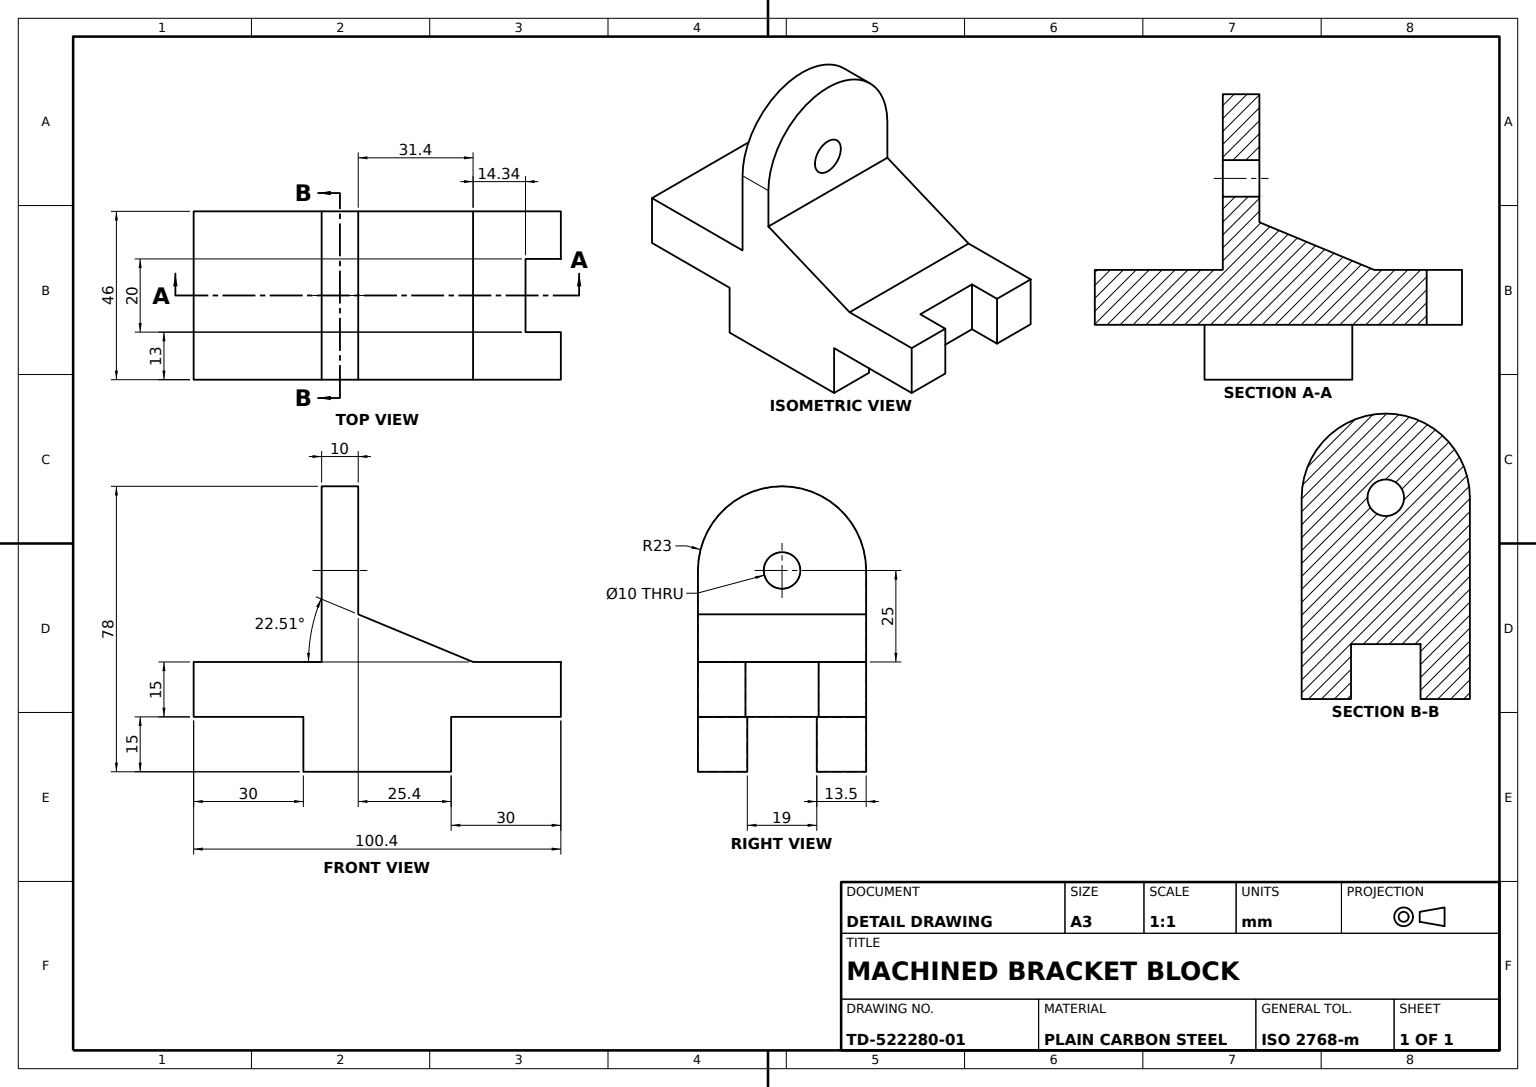
SolidWorks part; units mm, degrees
material "Plain Carbon Steel"
ref_plane "Front Plane" through (0, 0, 0) normal (0, 0, 1) x (1, 0, 0)
ref_plane "Top Plane" through (0, 0, 0) normal (0, 1, 0) x (1, 0, 0)
ref_plane "Right Plane" through (0, 0, 0) normal (1, 0, 0) x (0, 0, -1)
sketch "Base Profile Sketch" plane through (0, 0, 0) normal (1, 0, 0) x (0, 0, -1)
  line L0 (50.2023, 0) -> (-50.2023, 0)
  line L1 (-50.2023, 0) -> (-50.2023, -15)
  line L2 (-50.2023, -15) -> (-20.2023, -15)
  line L3 (-20.2023, -15) -> (-20.2023, -30)
  line L4 (50.2023, 0) -> (50.2023, -15)
  line L5 (50.2023, -15) -> (20.2023, -15)
  line L6 (20.2023, -15) -> (20.2023, -30)
  line L7 (20.2023, -30) -> (-20.2023, -30)
  point P4 (0, 0)
  dimension "D1" = 15
  dimension "D2" = 30
  dimension "D3" = 15
  dimension "D4" = 15
  dimension "D5" = 30
  dimension "D6" = 100.4046
extrude "Base Body" add sketch "Base Profile Sketch" along normal blind 46
ref_plane "Plane1" through (23, 0, 0) normal (1, 0, 0) x (0, 0, -1)
sketch "Side Block Sketch" plane through (23, 0, 0) normal (1, 0, 0) x (0, 0, -1)
  line L9 (-5.2023, 0) -> (-15.2023, 0)
  line L10 (-5.2023, 0) -> (-5.2023, 25)
  line L11 (-15.2023, 0) -> (-15.2023, 25)
  line L12 (-5.2023, 25) -> (-15.2023, 25)
  dimension "D1" = 10
  dimension "D2" = 25
  dimension "D3" = 5.2023
ref_plane "Plane2" through (23, 0, 0) normal (-1, 0, 0) x (0, 0, 1)
extrude "Side Block" add sketch "Side Block Sketch" along normal mid plane 46
sketch "Front Block Sketch" plane through (23, 0, 0) normal (1, 0, 0) x (0, 0, -1)
  line L0 (50.2023, 0) -> (-5.2023, 0) construction
  line L3 (-5.2023, 13.0152) -> (26.2023, 0)
  line L4 (26.2023, 0) -> (-5.2023, 0)
  line L7 (-5.2023, 13) -> (-5.2023, 0)
  line L8 (-5.2023, 0) -> (-5.2023, 25) construction
  line L9 (-5.2023, 13) -> (-5.2023, 13.0152)
  dimension "D1" = 31.4046
  dimension "D2" = 0.0152
  dimension "D3" = 13.0152
extrude "Front Block" add sketch "Front Block Sketch" along normal mid plane 46
sketch "Lug Sketch" plane through (0, 0, 5.2023) normal (0, 0, -1) x (-1, 0, 0)
  line L0 (-46, 25) -> (0, 25) construction
  line L1 (-46, 25) -> (0, 25)
  arc A0 (0, 25) -> (-46, 25) centre (-23, 25) ccw
  circle A1 centre (-23, 25) radius 10
  line M4 (0, 25) -> (-46, 25)
  dimension "D1" = 20
extrude "Lug" add sketch "Lug Sketch" against normal blind 10 contours A1 A0 M4
sketch "Lug Extension Sketch" plane through (0, 0, 5.2023) normal (0, 0, -1) x (-1, 0, 0)
  line L0 (-33, 25) -> (-13, 25) construction
  line L1 (-33, 25) -> (-13, 25)
  circle A0 centre (-23, 25) radius 5
  arc A1 (-13, 25) -> (-33, 25) centre (-23, 25) ccw construction
  arc A2 (-13, 25) -> (-33, 25) centre (-23, 25) ccw
  arc M1 (-33, 25) -> (-13, 25) centre (-23, 25) cw
  line M2 (-13, 25) -> (-33, 25)
  dimension "D1" = 10
extrude "Lug Extension" add sketch "Lug Extension Sketch" against normal blind 10 contours A0 M2 M1 | L1 A0
sketch "Pin Hole Sketch" plane through (0, 0, 5.2023) normal (0, 0, -1) x (-1, 0, 0)
  circle A0 centre (-23, 25) radius 5
  dimension "D1" = 10
extrude "Lug Pin Hole" cut sketch "Pin Hole Sketch" against normal blind 10
sketch "Slot Sketch" plane through (0, 0, 0) normal (0, 1, 0) x (1, 0, 0)
  line L0 (46, 50.2023) -> (0, 50.2023) construction
  line L1 (33, 59.8639) -> (13, 59.8639)
  line L2 (33, 59.8639) -> (33, 40.5407)
  line L3 (33, 40.5407) -> (13, 40.5407)
  line L4 (13, 59.8639) -> (13, 40.5407)
  line L5 (33, 59.8639) -> (13, 40.5407) construction
  line L6 (33, 40.5407) -> (13, 59.8639) construction
  line L8 (46, 26.2023) -> (0, 26.2023) construction
  point P0 (23, 50.2023)
  dimension "D1" = 20
  dimension "D2" = 14.3384
extrude "Slot Cut" cut sketch "Slot Sketch" against normal blind 19
sketch "Angled Cut Sketch" plane through (0, 0, -20.2023) normal (0, 0, -1) x (-1, 0, 0)
  line L0 (-23, -15) -> (-32.5, -15)
  line L1 (-13, -15) -> (-33, -15) construction
  line L2 (0, -30) -> (0, -15) construction
  line L3 (-46, -15) -> (0, -15) construction
  line L4 (-23, -15) -> (-13.5, -15)
  line L5 (-13.5, -15) -> (-13.5, -32.2148)
  line L6 (-13.5, -32.2148) -> (-32.5, -32.2148)
  line L7 (-32.5, -32.2148) -> (-32.5, -15)
  point P3 (-23, -15)
  dimension "D1" = 13.5
  dimension "D2" = 17.2148
extrude "Angled Relief Cut" cut sketch "Angled Cut Sketch" against normal blind 81
